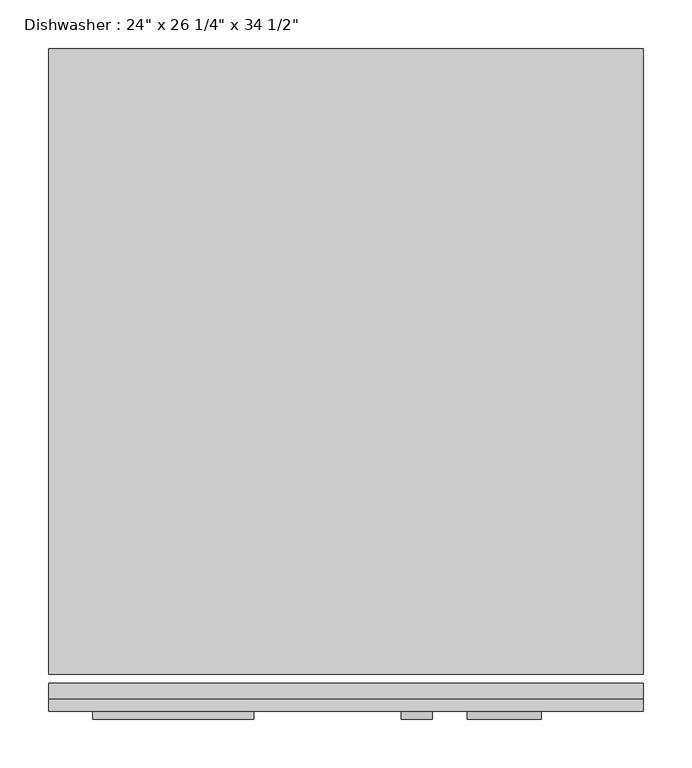
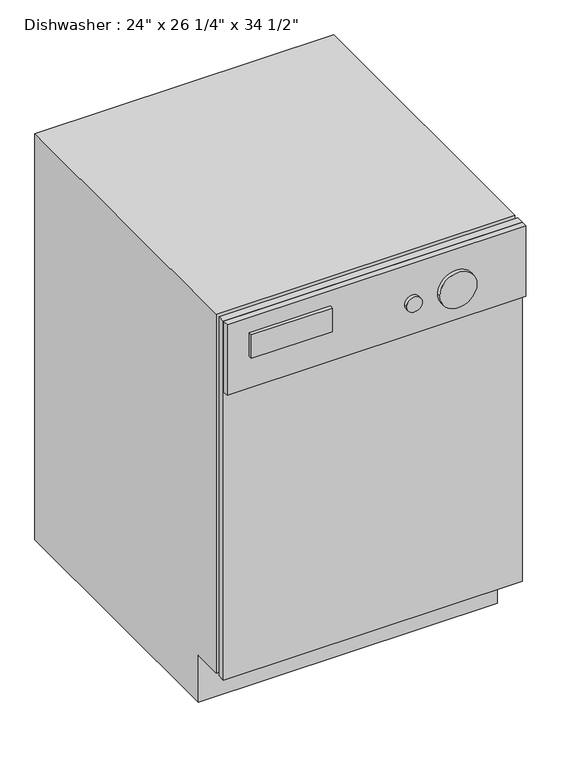
"""IFC4 building model written with IfcOpenShell, lengths in millimetres: proxy geometry."""

from ifc_helpers import new_model, si_unit, point, frame, frame_2d, origin, place, context, project, spatial, polyline, circle_curve, trimmed, segment, composite_curve, outline, extrude, source, transform, mapped, element, save


def proxy_19aded4c(model_context):
    return source(origin(), model_context, "Body", "SweptSolid", [
        extrude(outline(polyline([(687.1174685, -38.3504352), (77.5174685, -38.3504352), (77.5174685, -22.4754352), (687.1174685, -22.4754352), (687.1174685, -38.3504352)])), frame((0.0, 0.0, 101.6), z_axis=(0.0, 0.0, 1.0), x_axis=(1.0, 0.0, 0.0)), (0.0, 0.0, 1.0), 774.7),
        extrude(outline(polyline([(687.1174685, -38.3504352), (687.1174685, -51.0504352), (77.5174685, -51.0504352), (77.5174685, -38.3504352), (687.1174685, -38.3504352)])), frame((0.0, 0.0, 723.9), z_axis=(0.0, 0.0, 1.0), x_axis=(1.0, 0.0, 0.0)), (0.0, 0.0, 1.0), 152.4),
        extrude(outline(polyline([(628.3995648, 0.0), (50.5495648, 0.0), (50.5495648, 101.6), (-12.9504352, 101.6), (-12.9504352, 876.3), (628.3995648, 876.3), (628.3995648, 0.0)])), frame((77.5174685, 0.0, 0.0), z_axis=(1.0, 0.0, 0.0), x_axis=(0.0, 1.0, 0.0)), (0.0, 0.0, 1.0), 609.6),
        extrude(outline(polyline([(287.6378068, -59.1863727), (122.5378068, -59.1863727), (122.5378068, -51.0504352), (287.6378068, -51.0504352), (287.6378068, -59.1863727)])), frame((0.0, 0.0, 792.7846419), z_axis=(0.0, 0.0, 1.0), x_axis=(1.0, 0.0, 0.0)), (0.0, 0.0, 1.0), 50.8),
        extrude(outline(composite_curve([segment(trimmed(circle_curve(frame_2d((792.7846419, 544.7247133)), 38.1), [point((792.7846419, 506.6247133))], [point((792.7846419, 582.8247133))], False, "CARTESIAN"), True, "CONTINUOUS"), segment(trimmed(circle_curve(frame_2d((792.7846419, 544.7247133)), 38.1), [point((792.7846419, 582.8247133))], [point((792.7846419, 506.6247133))], False, "CARTESIAN"), True, "CONTINUOUS")], self_intersect=False)), frame((0.0, -59.1863727, 0.0), z_axis=(0.0, 1.0, 0.0), x_axis=(0.0, 0.0, 1.0)), (0.0, 0.0, 1.0), 8.1359375),
        extrude(outline(composite_curve([segment(trimmed(circle_curve(frame_2d((792.7846419, 455.195318)), 15.875), [point((792.7846419, 439.320318))], [point((792.7846419, 471.070318))], False, "CARTESIAN"), True, "CONTINUOUS"), segment(trimmed(circle_curve(frame_2d((792.7846419, 455.195318)), 15.875), [point((792.7846419, 471.070318))], [point((792.7846419, 439.320318))], False, "CARTESIAN"), True, "CONTINUOUS")], self_intersect=False)), frame((0.0, -59.1863727, 0.0), z_axis=(0.0, 1.0, 0.0), x_axis=(0.0, 0.0, 1.0)), (0.0, 0.0, 1.0), 8.1359375),
    ])


if __name__ == "__main__":
    model = new_model("IFC4")
    model_context = context("Model", 3, world=origin())
    ifc_project = project(units=[si_unit("LENGTHUNIT", "METRE", prefix="MILLI")], contexts=[model_context])
    site = spatial("IfcSite", under=ifc_project)
    building = spatial("IfcBuilding", under=site)
    placement = place(None, origin())
    proxy_shape = proxy_19aded4c(model_context)
    element("IfcBuildingElementProxy", 1, Name="Dishwasher : 24\" x 26 1/4\" x 34 1/2\"", ObjectType="Dishwasher : 24\" x 26 1/4\" x 34 1/2\"", at=placement, inside=building, context=model_context, shape_type="MappedRepresentation", body=[
        mapped(proxy_shape, transform((0.0, 0.0, 0.0), x_axis=(1.0, 0.0, 0.0), y_axis=(0.0, 1.0, 0.0), z_axis=(0.0, 0.0, 1.0))),
    ])
    save(model, "model.ifc")

# Revit data of these elements
# Type "Dishwasher : 24\" x 26 1/4\" x 34 1/2\""
#   Label = "DW"
#   Assembly Code = "E1090400"
#   Depth = 2' - 2 1/4"
#   Height = 2' - 10 1/2"
#   Width = 2' - 0"
#   Dishwasher Material = Steel, Paint Finish, Ivory, Glossy
#   Panel Face Material = Plastic, Opaque Black
#   Default Elevation = 0
# Element 1 (IfcBuildingElementProxy, "Dishwasher : 24\" x 26 1/4\" x 34 1/2\"")
#   Materials on its faces: "Steel, Paint Finish, Ivory, Glossy", "Plastic, Opaque Black"
# Materials
#   "Steel, Paint Finish, Ivory, Glossy": class "Metal", colour RGB 247 247 239, transparency 0, Description = "Steel, paint finish, ivory, glossy", Cost = 0
#   "Plastic, Opaque Black": class "Plastic", colour RGB 0 0 0, transparency 0.7, Description = "Plastic, generic, opaque black", Cost = 0
